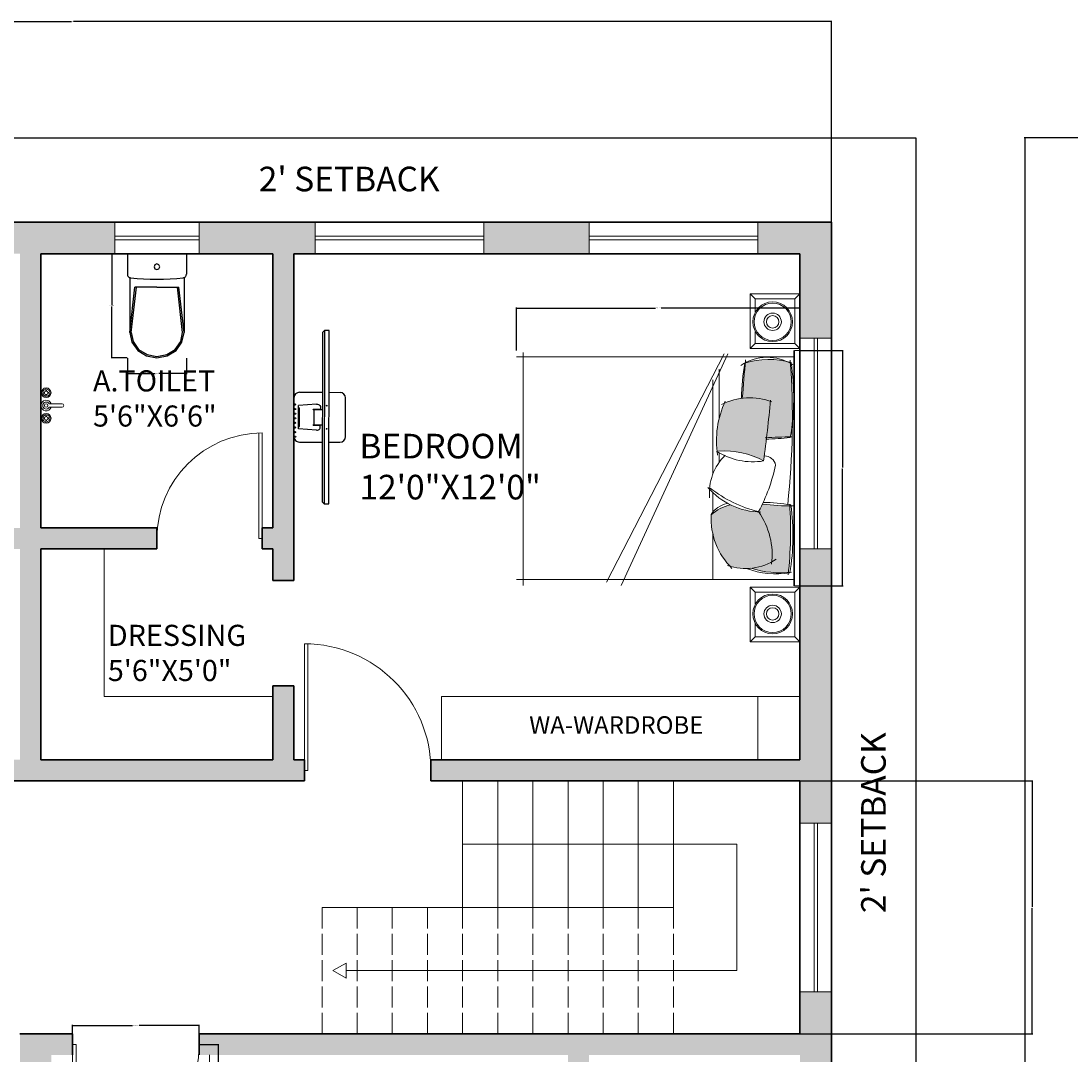
# Model space of a CAD drawing. Units: inches. Extents: x 3386 to 4477, y 1118 to 1824.
# Tile 5 of 7: x 3645 to 3944, y 1530 to 1824. Entities that reach past the tile are written whole.
import ezdxf

# ---------------------------------------------------------------- set-up
doc = ezdxf.new("R2010")
doc.units = ezdxf.units.IN
doc.linetypes.add('ACAD_ISO02W100', pattern=[15, 12, -3])
for name, color, linetype, lineweight in [('0.10', 252, 'Continuous', 9), ('0.15', 34, 'Continuous', 15), ('A-ANNO-DIMS', 2, 'Continuous', 18), ('A-ANNO-SYMB', 7, 'Continuous', 18), ('A-ANNO-TEXT', 7, 'Continuous', 18), ('A-AREA-IDEN', 7, 'Continuous', 18), ('A-DOOR', 4, 'Continuous', 18), ('A-EQPM', 9, 'Continuous', 18), ('A-FLOR-CASE', 7, 'Continuous', 18), ('A-FLOR-STRS', 7, 'Continuous', 18), ('A-FLOR-STRS-HIDN', 7, 'ACAD_ISO02W100', 13), ('A-FURN', 8, 'Continuous', 18), ('A-GLAZ', 4, 'Continuous', 18), ('A-WALL', 7, 'Continuous', 35), ('C-PROP', 7, 'Continuous', 25), ('Сантехника', 7, 'Continuous', 18)]:
    doc.layers.add(name, color=color, linetype=linetype, lineweight=lineweight)
doc.layers.add('A-FURN-PATT', color=116, linetype='Continuous', lineweight=13, true_color=0x136734)
doc.layers.add('A-WALL-PATT', color=18, linetype='Continuous', lineweight=13, true_color=0x000000)
doc.layers.add('SANTEH', color=7, linetype='Continuous')
doc.layers.add('window', color=130, linetype='Continuous')
doc.styles.get("Standard").update_dxf_attribs({"font": 'arial.ttf'})
doc.dimstyles.get("Standard").update_dxf_attribs({"dimtxt": 0.18, "dimasz": 0.18, "dimexe": 0.18, "dimexo": 0.0625, "dimgap": 0.09, "dimtad": 0, "dimtih": 1, "dimtoh": 1, "dimdec": 4, "dimzin": 0, "dimdsep": 46, "dimtxsty": 'Standard', "dimcen": 0.09, "dimadec": 0, "dimazin": 0, "dimtfac": 1, "dimtdec": 4, "dimtofl": 0, "dimtmove": 0, "dimatfit": 3, "dimfxl": 1, "dimtolj": 1, "dimtzin": 0, "dimarcsym": 0})

# ---------------------------------------------------------------- blocks, each defined once
blk = doc.blocks.new('D1')
for p, q in [((0, 36), (0, 0)), ((1, 36), (1, 0)), ((0, 0), (1, 0))]:
    blk.add_line(p, q)
blk.add_arc((0, 0), 36, 0, 90)
blk = doc.blocks.new('D2')
for p, q in [((0, 30), (0, 0)), ((1, 30), (1, 0)), ((0, 0), (1, 0))]:
    blk.add_line(p, q)
blk.add_arc((0, 0), 30, 0, 90)
blk = doc.blocks.new('WC 2 Symb_109')
at = {"layer": 'SANTEH'}
for p, q in [((0, 0), (0, 380)), ((0, 380), (132.4, 380)), ((153.6, 364.9), (506.8, 364.9)), ((506.3, 364.9), (215.7, 330.9)), ((506.3, 356), (215.7, 322)), ((215.7, 190), (215.7, 330.9)), ((215.7, 190), (215.7, 49.1)), ((153.8, 15.1), (506.8, 15.1)), ((506.3, 24), (215.7, 58)), ((506.3, 15.1), (215.7, 49.1)), ((0, 0), (132.4, 0))]:
    blk.add_line(p, q, dxfattribs=at)
for points in [[(154.6, 360.1), (153.9, 364.1), (152.3, 367.9), (150.2, 371.3), (147.4, 374.3), (144.1, 376.7), (140.5, 378.5), (136.5, 379.6), (132.4, 380)], [(154.6, 19.7), (158.6, 62.1), (161.4, 104.7), (163.1, 147.3), (163.7, 189.9), (163.1, 232.5), (161.4, 275.1), (158.6, 317.7), (154.6, 360.1)], [(506.3, 24), (565.5, 36.6), (615.7, 72.6), (649.2, 126.5), (661, 190), (649.2, 253.5), (615.7, 307.4), (565.5, 343.4), (506.3, 356)], [(506.8, 15.1), (569.2, 28.4), (622.2, 66.3), (657.6, 123.1), (670, 190), (657.6, 256.9), (622.2, 313.7), (569.2, 351.6), (506.8, 364.9)], [(132.4, 0), (136.5, 0.4), (140.4, 1.5), (144.1, 3.2), (147.3, 5.6), (150.1, 8.6), (152.3, 12), (153.8, 15.7), (154.6, 19.7)]]:
    blk.add_lwpolyline(points, dxfattribs=at)
blk.add_lwpolyline([(83.6, 208.5), (70.4, 203.1), (64.9, 190), (70.4, 176.9), (83.6, 171.5), (96.8, 176.9), (102.2, 190), (96.8, 203.1)], close=True, dxfattribs=at)
blk = doc.blocks.new('Faucet - Bathroom top')
for p, q in [((-4.107, 0.125), (-4.375, 0.125)), ((-3.75, 0.4788), (-3.75, 0.75)), ((-3.5, 0.482), (-3.5, 0.75)), ((-3.1461, 0.125), (-2.875, 0.125)), ((3.143, 0.125), (2.875, 0.125)), ((3.5, 0.4788), (3.5, 0.75)), ((3.75, 0.482), (3.75, 0.75)), ((4.1039, 0.125), (4.375, 0.125)), ((-4.1039, -0.125), (-4.375, -0.125)), ((-3.75, -0.4821), (-3.75, -0.75)), ((-3.5, -0.4789), (-3.5, -0.75)), ((-3.143, -0.125), (-2.875, -0.125)), ((-0.5, -0.8639), (-0.5, -4.5)), ((0.5, -4.5), (0.5, -0.8631)), ((3.1461, -0.125), (2.875, -0.125)), ((3.5, -0.4821), (3.5, -0.75)), ((3.75, -0.4789), (3.75, -0.75)), ((4.107, -0.125), (4.375, -0.125))]:
    blk.add_line(p, q)
for centre, radius in [((-3.625, 0), 1.375), ((-4.625, 0), 0.2795), ((-3.625, 0), 0.5), ((-3.625, 1), 0.2795), ((-2.625, 0), 0.2795), ((0, 0), 0.5), ((3.625, 0), 1.375), ((2.625, 0), 0.2795), ((3.625, 0), 0.5), ((3.625, 1), 0.2795), ((4.625, 0), 0.2795), ((-3.625, -1), 0.2795), ((3.625, -1), 0.2795)]:
    blk.add_circle(centre, radius)
for centre, radius, start, end in [((-3.625, 0), 1, 105.2407, 164.2093), ((-3.625, 0), 1, 16.44125, 74.07887), ((0, 0), 1.5, 289.6514, 250.3603), ((0, 0), 1, 300.3431, 239.7554), ((3.625, 0), 1, 106.12, 164.0884), ((3.625, 0), 1, 16.23422, 73.90469), ((-3.625, 0), 1, 196.2342, 253.9047), ((-3.625, 0), 1, 286.12, 344.0884), ((3.625, 0), 1, 196.4413, 254.0789), ((3.625, 0), 1, 285.2407, 344.2093), ((0, -4.5), 0.5, 180, 0)]:
    blk.add_arc(centre, radius, start, end)
blk = doc.blocks.new('TV')
at = {"color": 0}
for p, q in [((3967.27, 1784.85), (3967.05, 1784.65)), ((3967.76, 1763.68), (3967.54, 1763.86))]:
    blk.add_line(p, q, dxfattribs=at)
at = {"layer": 'window'}
for p, q in [((3967.54, 1763.86), (3967.05, 1784.65)), ((3964.41, 1777.23), (3967.22, 1777.3)), ((3968.01, 1777.32), (3969.36, 1777.35)), ((3966.53, 1775.82), (3964.33, 1775.61)), ((3964.34, 1775.34), (3964.45, 1775.34)), ((3964.34, 1775.31), (3964.43, 1775.32)), ((3966.14, 1775.2), (3967.01, 1775.22)), ((3966.14, 1775.18), (3967.27, 1775.2)), ((3966.14, 1775.18), (3966.14, 1775.2)), ((3966.3, 1773.29), (3966.26, 1775.18)), ((3964.39, 1773.06), (3964.48, 1773.06)), ((3966.19, 1773.28), (3967.31, 1773.31)), ((3966.19, 1773.26), (3967.05, 1773.28)), ((3966.19, 1773.26), (3966.19, 1773.28)), ((3964.39, 1773.04), (3964.5, 1773.04)), ((3966.61, 1772.66), (3964.4, 1772.77)), ((3964.55, 1771.15), (3967.36, 1771.22)), ((3968.15, 1771.24), (3969.5, 1771.27))]:
    blk.add_line(p, q, dxfattribs=at)
for points in [[(3968.33, 1763.69), (3967.83, 1784.86), (3967.27, 1784.85), (3967.76, 1763.68), (3968.33, 1763.69)], [(3963.86, 1771.81), (3963.75, 1776.54)], [(3970.16, 1771.96), (3970.05, 1776.69)], [(3964.4, 1772.77), (3964.33, 1775.61)], [(3964.48, 1773.06), (3964.43, 1775.32)], [(3964.5, 1773.04), (3964.45, 1775.34)]]:
    blk.add_lwpolyline(points, dxfattribs=at)
for points in [[(3966.53, 1775.82, -0.263666), (3966.93, 1775.69), (3967, 1775.57), (3967.01, 1775.22)], [(3966.61, 1772.66, 0.263666), (3967, 1772.81), (3967.06, 1772.93), (3967.05, 1773.28)]]:
    blk.add_lwpolyline(points, format="xyb", dxfattribs=at)
for centre, radius in [((3963.91, 1775.73), 0.0679), ((3967.77, 1775.68), 0.0451), ((3963.93, 1775.17), 0.0679), ((3963.94, 1774.6), 0.0679), ((3963.95, 1774.04), 0.0679), ((3963.97, 1773.48), 0.0679), ((3963.98, 1772.92), 0.0679), ((3963.99, 1772.35), 0.0679), ((3964.01, 1771.79), 0.0679), ((3967.83, 1772.86), 0.0451)]:
    blk.add_circle(centre, radius, dxfattribs=at)
for centre, start, end in [((3964.42, 1776.56), 91.3414, 181.3414), ((3969.38, 1776.67), 1.3414, 91.3414), ((3964.53, 1771.83), 181.3414, 271.3414), ((3969.49, 1771.94), 271.3414, 1.3414)]:
    blk.add_arc(centre, 0.676, start, end, dxfattribs=at)
blk = doc.blocks.new('camita')
at = {"layer": '0.10'}
for p, q in [((-0.85, -0.045), (0.85, -0.045)), ((-0.805, -0.045), (-0.805, -2.0485)), ((0.805, -0.045), (0.805, -2.0485)), ((-0.8271, -0.521), (0.8464, -1.2932)), ((-0.8271, -0.5476), (0.8236, -1.3992)), ((-0.7161, -0.585), (-0.3554, -0.585)), ((-0.1136, -0.585), (-0.0485, -0.585)), ((-0.638, -0.63), (0.0434, -0.63)), ((0.1749, -0.63), (0.3179, -0.63)), ((0.4739, -0.63), (0.805, -0.63)), ((-0.8354, -2), (0.8464, -2))]:
    blk.add_line(p, q, dxfattribs=at)
blk.add_lwpolyline([(-0.85, -0.0405), (0.85, -0.0405), (0.85, 0), (-0.85, 0)], close=True, dxfattribs=at)
for centre, radius, start, end in [((-0.4574, -0.2364), 0.3443, 147.50996, 213.83359), ((-0.1997, -0.2266), 0.5864, 163.92635, 197.14087), ((-0.3639, -5.8457), 5.7909, 83.80731, 94.12107), ((-0.5104, -1.7232), 1.6781, 80.12554, 98.66187), ((2.3534, -0.0532), 2.5803, 180.10628, 184.38541), ((-1.5443, -0.2452), 1.3333, 359.93941, 7.55329), ((1.5815, -0.2893), 1.3353, 170.38021, 178.99138), ((-1.4396, -0.0609), 1.7117, 352.92911, 0.39592), ((0.4524, -3.0675), 2.9996, 83.90257, 93.67595), ((0.4863, -1.6286), 1.5781, 80.16015, 98.05996), ((0.0294, -0.1377), 0.7262, 342.58415, 6.00484), ((0.1326, -0.1696), 0.6307, 339.92303, 8.74334), ((-0.0543, -0.3633), 0.4542, 159.30257, 206.50263), ((-1.3301, -9.6748), 9.4985, 82.27078, 84.93989), ((-0.007, -0.258), 0.0828, 100.01798, 179.73597), ((-0.2931, -1.4378), 1.2903, 61.97485, 77.84351), ((0.6265, -0.7518), 0.5508, 82.96906, 124.67388), ((0.3203, -0.3944), 0.4043, 341.45245, 33.45121), ((0.4585, -0.5454), 0.5842, 151.04555, 184.14969), ((-0.5341, -0.3393), 0.4875, 327.26442, 9.0473), ((-0.1986, -0.2742), 0.5159, 310.73945, 359.05759), ((-0.5673, -0.0868), 0.9057, 321.69527, 346.46261), ((-1.8672, -14.986), 14.6323, 84.65974, 85.75157), ((-0.4598, 1.4861), 1.9092, 260.95299, 268.65169), ((0.4384, -0.4834), 0.1898, 193.68485, 236.70352), ((0.5707, -0.4317), 0.3145, 192.93877, 221.96363), ((0.3612, -0.133), 0.5096, 267.25889, 315.29965), ((-0.2002, 0.064), 0.6673, 244.78094, 279.06058), ((0.179, -0.272), 0.3828, 224.52836, 275.22287)]:
    blk.add_arc(centre, radius, start, end, dxfattribs=at)
blk = doc.blocks.new('VELADOR')
at = {"layer": '0.15'}
for p, q in [((-0.2475, 0), (-0.2025, -0.045)), ((0.2475, 0), (0.2025, -0.045)), ((-0.2025, -0.405), (-0.2475, -0.45)), ((0.2475, -0.45), (0.2025, -0.405))]:
    blk.add_line(p, q, dxfattribs=at)
blk.add_lwpolyline([(-0.2475, 0), (-0.2475, -0.45), (0.2475, -0.45), (0.2475, 0)], close=True, dxfattribs=at)
blk.add_lwpolyline([(0.0921, -0.405), (0.2025, -0.405), (0.2025, -0.045), (-0.2025, -0.045), (-0.2025, -0.405), (-0.0818, -0.405)], dxfattribs=at)
for radius in [0.18, 0.1688, 0.0788, 0.0563]:
    blk.add_circle((0.0052, -0.2474), radius, dxfattribs=at)
blk = doc.blocks.new('WIN-24IN')
for p, q in [((0, 0), (0, 9)), ((24, 0), (24, 9)), ((0, 5), (24, 5)), ((0, 4), (24, 4))]:
    blk.add_line(p, q)
blk = doc.blocks.new('WIN-48IN')
for p, q in [((0, 48), (9, 48)), ((4, 0), (4, 48)), ((5, 0), (5, 48)), ((0, 0), (9, 0))]:
    blk.add_line(p, q)
blk = doc.blocks.new('WIN-60IN')
for p, q in [((0, 60), (9, 60)), ((4, 60), (4, 0)), ((5, 60), (5, 0)), ((0, 0), (9, 0))]:
    blk.add_line(p, q)
blk = doc.blocks.new('STAIR-DIRECTION')
blk.add_lwpolyline([(36.88, 38.16), (114.88, 38.16), (114.88, 2.16), (3.74, 2.16)])
blk.add_lwpolyline([(0, 2.16), (3.74, 0), (3.74, 4.32)], close=True)
blk = doc.blocks.new('WARDROBE-102IN')
for q in [(0, 18), (102, 0)]:
    blk.add_line((0, 0), q)
blk = doc.blocks.new('WARDROBE-102IN-DIVIDED')
for p, q in [((0, 18), (102, 18)), ((0, 0), (0, 18)), ((90, 18), (90, 0))]:
    blk.add_line(p, q)
blk = doc.blocks.new('DRESSING-UNIT-48X42')
for q in [(0, 42), (48, 0)]:
    blk.add_line((0, 0), q)
blk = doc.blocks.new('*D65')
at = {"layer": 'A-ANNO-DIMS', "color": 0, "lineweight": -2, "transparency": 16777216}
for p, q in [((3659.66, 1532.93), (3659.66, 1538.45)), ((3659.84, 1538.27), (3676.72, 1538.27)), ((3695.48, 1538.27), (3678.59, 1538.27)), ((3695.66, 1532.93), (3695.66, 1538.45))]:
    blk.add_line(p, q, dxfattribs=at)
at = {"layer": 'A-ANNO-DIMS', "color": 0, "transparency": 16777216}
for points in [[(3659.84, 1538.3), (3659.84, 1538.24), (3659.66, 1538.27)], [(3695.48, 1538.3), (3695.48, 1538.24), (3695.66, 1538.27)]]:
    blk.add_solid(points, dxfattribs=at)
at = {"layer": 'Defpoints', "color": 0, "transparency": 16777216}
for p in [(3695.66, 1538.27), (3659.66, 1532.87), (3695.66, 1532.87)]:
    blk.add_point(p, dxfattribs=at)
at = {"layer": 'A-ANNO-DIMS', "color": 0, "transparency": 16777216, "insert": (3677.66, 1538.27), "char_height": 0.18, "attachment_point": 5}
blk.add_mtext('\\A1;DOOR 36 TYP.', dxfattribs=at)
blk = doc.blocks.new('*D66')
at = {"layer": 'A-ANNO-DIMS', "color": 0, "lineweight": -2, "transparency": 16777216}
for p, q in [((3695.72, 1532.87), (3701.24, 1532.87)), ((3701.06, 1532.69), (3701.06, 1515.05)), ((3701.06, 1497.05), (3701.06, 1514.69)), ((3695.72, 1496.87), (3701.24, 1496.87))]:
    blk.add_line(p, q, dxfattribs=at)
at = {"layer": 'A-ANNO-DIMS', "color": 0, "transparency": 16777216}
for points in [[(3701.03, 1532.69), (3701.09, 1532.69), (3701.06, 1532.87)], [(3701.03, 1497.05), (3701.09, 1497.05), (3701.06, 1496.87)]]:
    blk.add_solid(points, dxfattribs=at)
at = {"layer": 'Defpoints', "color": 0, "transparency": 16777216}
for p in [(3695.66, 1532.87), (3695.66, 1496.87), (3701.06, 1496.87)]:
    blk.add_point(p, dxfattribs=at)
at = {"layer": 'A-ANNO-DIMS', "color": 0, "transparency": 16777216, "insert": (3701.06, 1514.87), "char_height": 0.18, "attachment_point": 5}
blk.add_mtext('\\A1;36 TYP.', dxfattribs=at)
blk = doc.blocks.new('*D77')
at = {"layer": 'A-ANNO-DIMS', "color": 0, "lineweight": -2, "transparency": 16777216}
for p, q in [((3675.2, 1757.87), (3670.64, 1757.87)), ((3670.82, 1757.69), (3670.82, 1743.25)), ((3670.82, 1728.44), (3670.82, 1742.88)), ((3675.2, 1728.26), (3670.64, 1728.26))]:
    blk.add_line(p, q, dxfattribs=at)
at = {"layer": 'A-ANNO-DIMS', "color": 0, "transparency": 16777216}
for points in [[(3670.79, 1757.69), (3670.85, 1757.69), (3670.82, 1757.87)], [(3670.79, 1728.44), (3670.85, 1728.44), (3670.82, 1728.26)]]:
    blk.add_solid(points, dxfattribs=at)
at = {"layer": 'Defpoints', "color": 0, "transparency": 16777216}
for p in [(3675.26, 1757.87), (3670.82, 1728.26), (3675.26, 1728.26)]:
    blk.add_point(p, dxfattribs=at)
at = {"layer": 'A-ANNO-DIMS', "color": 0, "transparency": 16777216, "insert": (3670.82, 1743.06), "char_height": 0.18, "attachment_point": 5}
blk.add_mtext('\\A1;WC 30 TYP.', dxfattribs=at)
blk = doc.blocks.new('*D78')
at = {"layer": 'A-ANNO-DIMS', "color": 0, "lineweight": -2, "transparency": 16777216}
for p, q in [((3675.26, 1728.2), (3675.26, 1723.64)), ((3692.05, 1728.2), (3692.05, 1723.64)), ((3675.44, 1723.82), (3683.14, 1723.82)), ((3691.87, 1723.82), (3684.17, 1723.82))]:
    blk.add_line(p, q, dxfattribs=at)
at = {"layer": 'A-ANNO-DIMS', "color": 0, "transparency": 16777216}
for points in [[(3675.44, 1723.85), (3675.44, 1723.79), (3675.26, 1723.82)], [(3691.87, 1723.85), (3691.87, 1723.79), (3692.05, 1723.82)]]:
    blk.add_solid(points, dxfattribs=at)
at = {"layer": 'Defpoints', "color": 0, "transparency": 16777216}
for p in [(3675.26, 1728.26), (3692.05, 1728.26), (3692.05, 1723.82)]:
    blk.add_point(p, dxfattribs=at)
at = {"layer": 'A-ANNO-DIMS', "color": 0, "transparency": 16777216, "insert": (3683.66, 1723.82), "char_height": 0.18, "attachment_point": 5}
blk.add_mtext('\\A1;17 TYP.', dxfattribs=at)
blk = doc.blocks.new('*D83')
at = {"layer": 'A-ANNO-DIMS', "color": 0, "lineweight": -2, "transparency": 16777216}
for p, q in [((3786, 1730.37), (3786, 1742.58)), ((3786.18, 1742.4), (3825.51, 1742.4)), ((3866.48, 1742.4), (3827.14, 1742.4)), ((3866.66, 1730.37), (3866.66, 1742.58))]:
    blk.add_line(p, q, dxfattribs=at)
at = {"layer": 'A-ANNO-DIMS', "color": 0, "transparency": 16777216}
for points in [[(3786.18, 1742.43), (3786.18, 1742.37), (3786, 1742.4)], [(3866.48, 1742.43), (3866.48, 1742.37), (3866.66, 1742.4)]]:
    blk.add_solid(points, dxfattribs=at)
at = {"layer": 'Defpoints', "color": 0, "transparency": 16777216}
for p in [(3866.66, 1742.4), (3786, 1730.3), (3866.66, 1730.3)]:
    blk.add_point(p, dxfattribs=at)
at = {"layer": 'A-ANNO-DIMS', "color": 0, "transparency": 16777216, "insert": (3826.33, 1742.4), "char_height": 0.18, "attachment_point": 5}
blk.add_mtext('\\A1;BED 81 TYP.', dxfattribs=at)
blk = doc.blocks.new('*D84')
at = {"layer": 'A-ANNO-DIMS', "color": 0, "lineweight": -2, "transparency": 16777216}
for p, q in [((3866.72, 1730.3), (3878.93, 1730.3)), ((3878.75, 1730.12), (3878.75, 1697.02)), ((3878.75, 1663.55), (3878.75, 1696.65)), ((3866.72, 1663.37), (3878.93, 1663.37))]:
    blk.add_line(p, q, dxfattribs=at)
at = {"layer": 'A-ANNO-DIMS', "color": 0, "transparency": 16777216}
for points in [[(3878.72, 1730.12), (3878.78, 1730.12), (3878.75, 1730.3)], [(3878.72, 1663.55), (3878.78, 1663.55), (3878.75, 1663.37)]]:
    blk.add_solid(points, dxfattribs=at)
at = {"layer": 'Defpoints', "color": 0, "transparency": 16777216}
for p in [(3866.66, 1730.3), (3866.66, 1663.37), (3878.75, 1663.37)]:
    blk.add_point(p, dxfattribs=at)
at = {"layer": 'A-ANNO-DIMS', "color": 0, "transparency": 16777216, "insert": (3878.75, 1696.83), "char_height": 0.18, "attachment_point": 5}
blk.add_mtext('\\A1;67 TYP.', dxfattribs=at)
blk = doc.blocks.new('*D103')
at = {"layer": 'A-ANNO-DIMS', "color": 0, "lineweight": -2, "transparency": 16777216}
for p, q in [((3443.66, 1745.93), (3443.66, 1824.1)), ((3443.84, 1823.92), (3659.36, 1823.92)), ((3875.48, 1823.92), (3659.95, 1823.92)), ((3875.66, 1766.93), (3875.66, 1824.1))]:
    blk.add_line(p, q, dxfattribs=at)
at = {"layer": 'A-ANNO-DIMS', "color": 0, "transparency": 16777216}
for points in [[(3443.84, 1823.95), (3443.84, 1823.89), (3443.66, 1823.92)], [(3875.48, 1823.95), (3875.48, 1823.89), (3875.66, 1823.92)]]:
    blk.add_solid(points, dxfattribs=at)
at = {"layer": 'Defpoints', "color": 0, "transparency": 16777216}
for p in [(3875.66, 1823.92), (3875.66, 1766.87), (3443.66, 1745.87)]:
    blk.add_point(p, dxfattribs=at)
at = {"layer": 'A-ANNO-DIMS', "color": 0, "transparency": 16777216, "insert": (3659.66, 1823.92), "char_height": 0.18, "attachment_point": 5}
blk.add_mtext('\\A1;432', dxfattribs=at)
blk = doc.blocks.new('*D104')
at = {"layer": 'A-ANNO-DIMS', "color": 0, "lineweight": -2, "transparency": 16777216}
for p, q in [((3866.72, 1607.87), (3932.89, 1607.87)), ((3932.71, 1607.69), (3932.71, 1572.05)), ((3932.71, 1536.05), (3932.71, 1571.69)), ((3866.72, 1535.87), (3932.89, 1535.87))]:
    blk.add_line(p, q, dxfattribs=at)
at = {"layer": 'A-ANNO-DIMS', "color": 0, "transparency": 16777216}
for points in [[(3932.68, 1607.69), (3932.74, 1607.69), (3932.71, 1607.87)], [(3932.68, 1536.05), (3932.74, 1536.05), (3932.71, 1535.87)]]:
    blk.add_solid(points, dxfattribs=at)
at = {"layer": 'Defpoints', "color": 0, "transparency": 16777216}
for p in [(3866.66, 1607.87), (3932.71, 1607.87), (3866.66, 1535.87)]:
    blk.add_point(p, dxfattribs=at)
at = {"layer": 'A-ANNO-DIMS', "color": 0, "transparency": 16777216, "insert": (3932.71, 1571.87), "char_height": 0.18, "attachment_point": 5}
blk.add_mtext('\\A1;72', dxfattribs=at)
blk = doc.blocks.new('*D106')
at = {"layer": 'A-ANNO-DIMS', "color": 0, "lineweight": -2, "transparency": 16777216}
for p, q in [((3963.65, 1790.87), (3930.48, 1790.87)), ((3930.66, 1790.69), (3930.66, 1491.05)), ((3930.66, 1191.05), (3930.66, 1490.69)), ((3963.65, 1190.87), (3930.48, 1190.87))]:
    blk.add_line(p, q, dxfattribs=at)
at = {"layer": 'A-ANNO-DIMS', "color": 0, "transparency": 16777216}
for points in [[(3930.63, 1790.69), (3930.69, 1790.69), (3930.66, 1790.87)], [(3930.63, 1191.05), (3930.69, 1191.05), (3930.66, 1190.87)]]:
    blk.add_solid(points, dxfattribs=at)
at = {"layer": 'Defpoints', "color": 0, "transparency": 16777216}
for p in [(3930.66, 1790.87), (3963.71, 1790.87), (3963.71, 1190.87)]:
    blk.add_point(p, dxfattribs=at)
at = {"layer": 'A-ANNO-DIMS', "color": 0, "transparency": 16777216, "insert": (3930.66, 1490.87), "char_height": 0.18, "attachment_point": 5}
blk.add_mtext('\\A1;600', dxfattribs=at)

msp = doc.modelspace()

# ---------------------------------------------------------------- hatches: boundary and pattern name
at = {"layer": 'A-FURN-PATT'}
h = msp.add_hatch(color=256, dxfattribs=at)
h.dxf.hatch_style = 1
h.paths.add_polyline_path([(3850.23, 1716.73, -0.113891), (3858.22, 1715.87, -0.006967), (3857.15, 1705.5, -0.016701), (3863.93, 1705.77, 0.015442), (3864.5, 1709.81, 0.01851), (3863.97, 1726.68, 0.020657), (3862.97, 1727.18, 0.131047), (3851.08, 1726.81, -0.004387)])
h.paths.add_polyline_path([(3855.96, 1686.63, -0.011742), (3854.89, 1684.5, -0.175864), (3858.65, 1670.19, -0.098488), (3852.71, 1668.38, 0.094792), (3863.39, 1667.16, 0.040212), (3863.77, 1686.12, -0.029051)])
h = msp.add_hatch(color=256, dxfattribs=at)
h.dxf.hatch_style = 1
h.paths.add_polyline_path([(3845.14, 1715.39, -0.189536), (3858.22, 1715.91, -0.011408), (3856.31, 1698.95, 0.150361), (3843.07, 1701.73, -0.133776)])
h.paths.add_polyline_path([(3858.64, 1670.24, -0.194952), (3846.75, 1668.96, -0.202559), (3841.37, 1683.62, -0.127326), (3846.88, 1686.48, 0.104045), (3854.98, 1684.41, -0.173835)])
at = {"layer": 'A-WALL-PATT'}
h = msp.add_hatch(color=256, dxfattribs=at)
h.dxf.hatch_style = 1
h.paths.add_polyline_path([(3443.66, 1221.87), (3452.66, 1221.87), (3452.66, 1301.87), (3458.66, 1301.87), (3458.66, 1310.87), (3452.66, 1310.87), (3452.66, 1328.87), (3443.66, 1328.87)])
h.paths.add_polyline_path([(3506.66, 1310.87), (3506.66, 1306.37), (3506.66, 1301.87), (3530.66, 1301.87), (3530.66, 1310.87)])
h.paths.add_polyline_path([(3653.66, 1301.87), (3653.66, 1382.87), (3662.66, 1382.87), (3662.66, 1391.87), (3653.66, 1391.87), (3653.66, 1529.87), (3659.66, 1529.87), (3659.66, 1535.87), (3644.66, 1535.87), (3644.66, 1310.87), (3602.66, 1310.87), (3602.66, 1301.87)])
h.paths.add_polyline_path([(3452.66, 1406.87), (3443.66, 1406.87), (3443.66, 1376.87), (3452.66, 1376.87), (3452.66, 1388.44)])
h.paths.add_polyline_path([(3452.66, 1478.87), (3452.66, 1502.87), (3478.74, 1502.87), (3482.66, 1502.87), (3482.66, 1504.87), (3482.66, 1517.87), (3473.66, 1517.87), (3473.66, 1511.87), (3443.66, 1511.87), (3443.66, 1478.87)])
h.paths.add_polyline_path([(3773.66, 1391.87), (3710.66, 1391.87), (3710.66, 1382.87), (3773.66, 1382.87)], flags=17)
h.paths.add_polyline_path([(3824.66, 1391.87), (3806.66, 1391.87), (3806.66, 1469.87), (3809.66, 1469.87), (3809.66, 1472.87), (3809.66, 1475.87), (3806.66, 1475.87), (3806.66, 1478.87), (3800.66, 1478.87), (3800.66, 1463.32), (3800.66, 1391.87), (3797.66, 1391.87), (3797.66, 1382.87), (3824.66, 1382.87)], flags=17)
h.paths.add_polyline_path([(3866.66, 1469.87), (3866.66, 1391.87), (3848.66, 1391.87), (3848.66, 1382.87), (3875.66, 1382.87), (3875.66, 1547.87), (3866.66, 1547.87), (3866.66, 1535.87), (3695.66, 1535.87), (3695.66, 1529.87), (3800.66, 1529.87), (3800.66, 1508.87), (3806.66, 1508.87), (3806.66, 1529.87), (3866.66, 1529.87), (3866.66, 1475.87), (3839.66, 1475.87), (3839.66, 1469.87)])
h.paths.add_polyline_path([(3875.66, 1673.87), (3866.66, 1673.87), (3866.66, 1663.37), (3866.66, 1647.44), (3866.66, 1613.87), (3761.66, 1613.87), (3761.66, 1607.87), (3866.66, 1607.87), (3866.66, 1595.87), (3875.66, 1595.87)])
h.paths.add_polyline_path([(3473.66, 1607.87), (3473.66, 1601.87), (3482.66, 1601.87), (3482.66, 1616.87), (3452.66, 1616.87), (3452.66, 1640.87), (3443.66, 1640.87), (3443.66, 1607.87)])
h.paths.add_polyline_path([(3491.66, 1736.87), (3491.66, 1745.87), (3478.95, 1745.87), (3443.66, 1745.87), (3443.66, 1688.87), (3452.66, 1688.87), (3452.66, 1736.87)])
h.paths.add_polyline_path([(3551.66, 1745.87), (3539.66, 1745.87), (3539.66, 1736.87), (3551.66, 1736.87)])
h.paths.add_polyline_path([(3587.66, 1745.87), (3581.66, 1745.87), (3581.66, 1741.37), (3581.66, 1736.87), (3587.66, 1736.87), (3587.66, 1712.87), (3596.66, 1712.87), (3596.66, 1757.87), (3644.66, 1757.87), (3644.66, 1679.87), (3596.66, 1679.87), (3596.66, 1682.87), (3592.16, 1682.87), (3587.66, 1682.87), (3587.66, 1607.87), (3602.66, 1607.87), (3602.66, 1613.87), (3596.66, 1613.87), (3596.66, 1673.87), (3644.66, 1673.87), (3644.66, 1613.87), (3638.66, 1613.87), (3638.66, 1610.87), (3638.66, 1607.87), (3725.66, 1607.87), (3725.66, 1613.87), (3722.66, 1613.87), (3722.66, 1634.87), (3716.66, 1634.87), (3716.66, 1613.87), (3650.66, 1613.87), (3650.66, 1673.87), (3683.66, 1673.87), (3683.66, 1679.87), (3650.66, 1679.87), (3650.66, 1757.87), (3671.66, 1757.87), (3671.66, 1766.87), (3587.66, 1766.87)])
h.paths.add_polyline_path([(3716.66, 1757.87), (3716.66, 1679.87), (3713.66, 1679.87), (3713.66, 1673.87), (3716.66, 1673.87), (3716.66, 1664.87), (3722.66, 1664.87), (3722.66, 1757.87), (3728.66, 1757.87), (3728.66, 1766.87), (3695.66, 1766.87), (3695.66, 1757.87)])
h.paths.add_polyline_path([(3806.66, 1757.87), (3806.66, 1766.87), (3776.66, 1766.87), (3776.66, 1757.87)])
h.paths.add_polyline_path([(3875.66, 1766.87), (3854.66, 1766.87), (3854.66, 1757.87), (3866.66, 1757.87), (3866.66, 1733.87), (3875.66, 1733.87)])

# ---------------------------------------------------------------- linework, layer by layer
at = {"layer": 'A-FLOR-STRS'}
for p, q in [((3770.66, 1607.87), (3770.66, 1571.87)), ((3780.66, 1607.87), (3780.66, 1571.87)), ((3790.66, 1607.87), (3790.66, 1571.87)), ((3800.66, 1607.87), (3800.66, 1571.87)), ((3810.66, 1607.87), (3810.66, 1571.87)), ((3820.66, 1607.87), (3820.66, 1571.87)), ((3830.66, 1607.87), (3830.66, 1571.87)), ((3730.66, 1571.87), (3830.66, 1571.87))]:
    msp.add_line(p, q, dxfattribs=at)
at = {"layer": 'A-FLOR-STRS-HIDN', "ltscale": 0.5}
for p, q in [((3730.66, 1571.87), (3730.66, 1535.87)), ((3740.66, 1571.87), (3740.66, 1535.87)), ((3750.66, 1571.87), (3750.66, 1535.87)), ((3760.66, 1571.87), (3760.66, 1535.87)), ((3770.66, 1571.87), (3770.66, 1535.87)), ((3780.66, 1571.87), (3780.66, 1535.87)), ((3790.66, 1571.87), (3790.66, 1535.87)), ((3800.66, 1571.87), (3800.66, 1535.87)), ((3810.66, 1571.87), (3810.66, 1535.87)), ((3820.66, 1571.87), (3820.66, 1535.87)), ((3830.66, 1571.87), (3830.66, 1535.87))]:
    msp.add_line(p, q, dxfattribs=at)
at = {"layer": 'A-WALL'}
for p, q in [((3587.66, 1766.87), (3875.66, 1766.87)), ((3875.66, 1766.87), (3875.66, 1382.87)), ((3650.66, 1679.87), (3650.66, 1757.87)), ((3650.66, 1757.87), (3716.66, 1757.87)), ((3716.66, 1757.87), (3716.66, 1679.87)), ((3722.66, 1757.87), (3722.66, 1664.87)), ((3722.66, 1757.87), (3866.66, 1757.87)), ((3866.66, 1757.87), (3866.66, 1613.87)), ((3650.66, 1679.87), (3683.66, 1679.87)), ((3683.66, 1679.87), (3683.66, 1673.87)), ((3713.66, 1679.87), (3713.66, 1673.87)), ((3713.66, 1679.87), (3716.66, 1679.87)), ((3650.66, 1613.87), (3650.66, 1673.87)), ((3650.66, 1673.87), (3683.66, 1673.87)), ((3713.66, 1673.87), (3716.66, 1673.87)), ((3716.66, 1673.87), (3716.66, 1664.87)), ((3716.66, 1664.87), (3722.66, 1664.87)), ((3716.66, 1634.87), (3722.66, 1634.87)), ((3716.66, 1634.87), (3716.66, 1613.87)), ((3722.66, 1634.87), (3722.66, 1613.87)), ((3650.66, 1613.87), (3716.66, 1613.87)), ((3722.66, 1613.87), (3725.66, 1613.87)), ((3725.66, 1613.87), (3725.66, 1607.87)), ((3761.66, 1613.87), (3761.66, 1607.87)), ((3761.66, 1613.87), (3866.66, 1613.87)), ((3638.66, 1607.87), (3725.66, 1607.87)), ((3761.66, 1607.87), (3866.66, 1607.87)), ((3866.66, 1607.87), (3866.66, 1535.87)), ((3644.66, 1535.87), (3659.66, 1535.87)), ((3659.66, 1529.87), (3659.66, 1535.87)), ((3695.66, 1529.87), (3695.66, 1535.87)), ((3695.66, 1535.87), (3866.66, 1535.87))]:
    msp.add_line(p, q, dxfattribs=at)
at = {"layer": 'C-PROP'}
msp.add_lwpolyline([(3419.66, 1790.87), (3899.66, 1790.87), (3899.66, 1190.87), (3419.66, 1190.87)], close=True, dxfattribs=at)

# ---------------------------------------------------------------- block references
at = {"layer": 'A-ANNO-SYMB'}
msp.add_blockref('STAIR-DIRECTION', (3733.77, 1551.71), dxfattribs=at)
at = {"layer": 'A-DOOR', "xscale": -1}
msp.add_blockref('D2', (3713.66, 1676.87), dxfattribs=at)
at = {"layer": 'A-DOOR'}
msp.add_blockref('D1', (3725.66, 1610.87), dxfattribs=at)
at = {"layer": 'A-DOOR', "xscale": -1, "rotation": 180}
msp.add_blockref('D1', (3659.66, 1532.87), dxfattribs=at)
at = {"layer": 'A-EQPM', "xscale": 2.327319231123021, "yscale": 2.327319231123021, "zscale": 2.327319231123021, "rotation": 358.5430845181613}
msp.add_blockref('TV', (-5604.37, -2181.82), dxfattribs=at)
at = {"layer": 'A-FLOR-CASE'}
for name, p in [('DRESSING-UNIT-48X42', (3668.66, 1631.87)), ('WARDROBE-102IN-DIVIDED', (3764.66, 1613.87)), ('WARDROBE-102IN', (3698.66, 1511.87))]:
    msp.add_blockref(name, p, dxfattribs=at)
at = {"layer": 'A-FURN'}
for name, p, xscale, yscale, zscale, rotation in [('VELADOR', (3866.66, 1738.67), 31.41542173157097, 31.41542173157097, 31.41542173157097, 270), ('camita', (3866.66, 1696.83), 39.375, 39.375, 39.375, 270), ('VELADOR', (3866.66, 1655.22), -31.41542173157097, 31.41542173157097, 31.41542173157097, 269.9999999999999)]:
    msp.add_blockref(name, p, dxfattribs=dict(at, xscale=xscale, yscale=yscale, zscale=zscale, rotation=rotation))
at = {"layer": 'A-GLAZ'}
for name, p in [('WIN-24IN', (3671.66, 1757.87)), ('WIN-60IN', (3866.66, 1673.87)), ('WIN-48IN', (3866.66, 1547.87))]:
    msp.add_blockref(name, p, dxfattribs=at)
for p, rotation in [((3776.66, 1757.87), 89.99999999999818), ((3806.66, 1766.87), 269.9999999999999)]:
    msp.add_blockref('WIN-48IN', p, dxfattribs=dict(at, rotation=rotation))
at = {"layer": 'Сантехника', "xscale": 0.0441898926459964, "yscale": 0.0441898926459964, "zscale": 0.0441898926459964, "rotation": 269.9999999999999}
msp.add_blockref('WC 2 Symb_109', (3675.26, 1757.87), dxfattribs=at)
at = {"layer": 'Сантехника', "rotation": 90}
msp.add_blockref('Faucet - Bathroom top', (3652.16, 1714.68), dxfattribs=at)

# ---------------------------------------------------------------- texts
at = {"layer": 'A-ANNO-TEXT', "attachment_point": 1}
for s, insert, char_height in [("{\\fTimes New Roman|b0|i0|c0|p18;2' SETBACK}", (3712.65, 1782.64), 7), ('{\\fTimes New Roman|b0|i0|c0|p18;WA-WARDROBE}', (3789.61, 1626.26), 5)]:
    msp.add_mtext_dynamic_manual_height_columns(s, width=79.5604, gutter_width=12.5, heights=[0], dxfattribs=dict(at, insert=insert, char_height=char_height))
at = {"layer": 'A-ANNO-TEXT', "insert": (3884.07, 1570.24), "char_height": 7, "attachment_point": 1, "rotation": 90}
msp.add_mtext_dynamic_manual_height_columns("{\\fTimes New Roman|b0|i0|c0|p18;2' SETBACK}", width=79.5604, gutter_width=12.5, heights=[0], dxfattribs=at)
at = {"layer": 'A-AREA-IDEN', "attachment_point": 1}
for s, width, insert, char_height in [('{\\fTimes New Roman|b0|i0|c0|p18;A.TOILET\\P5\'6"X6\'6"}', 79.5604, (3665.48, 1724.69), 6), ('{\\fTimes New Roman|b0|i0|c0|p18;BEDROOM\\P12\'0"X12\'0"}', 79.5604, (3741.3, 1706.63), 7), ('{\\fTimes New Roman|b0|i0|c0|p18;DRESSING\\P5\'6"X5\'0"}', 52.5784, (3669.71, 1652.28), 6)]:
    msp.add_mtext_dynamic_manual_height_columns(s, width=width, gutter_width=12.5, heights=[0], dxfattribs=dict(at, insert=insert, char_height=char_height))

# ---------------------------------------------------------------- dimensions: what is measured, and where the dimension line sits
at = {"layer": 'A-ANNO-DIMS'}
dim = msp.add_linear_dim(base=(3875.66, 1823.92), p1=(3443.66, 1745.87), p2=(3875.66, 1766.87), dimstyle='Standard', override={"dimdec": 0, "dimlfac": 1, "dimrnd": 0, "dimzin": 0, "dimdsep": 46, "dimlunit": 2}, dxfattribs=at)
dim.commit()
dim.dimension.update_dxf_attribs({"geometry": '*D103', "text_midpoint": (3659.66, 1823.92)})
for base, p1, p2, picture, middle in [((3930.66, 1790.87), (3963.71, 1190.87), (3963.71, 1790.87), '*D106', (3930.66, 1490.87)), ((3932.71, 1607.87), (3866.66, 1535.87), (3866.66, 1607.87), '*D104', (3932.71, 1571.87))]:
    dim = msp.add_linear_dim(base=base, p1=p1, p2=p2, angle=90, dimstyle='Standard', override={"dimdec": 0, "dimlfac": 1, "dimrnd": 0, "dimzin": 0, "dimdsep": 46, "dimlunit": 2}, dxfattribs=at)
    dim.commit()
    dim.dimension.update_dxf_attribs({"geometry": picture, "text_midpoint": middle})
for base, p1, p2, text, picture, middle in [((3670.82, 1728.26), (3675.26, 1757.87), (3675.26, 1728.26), 'WC <> TYP.', '*D77', (3670.82, 1743.06)), ((3878.75, 1663.37), (3866.66, 1730.3), (3866.66, 1663.37), '<> TYP.', '*D84', (3878.75, 1696.83)), ((3701.06, 1496.87), (3695.66, 1532.87), (3695.66, 1496.87), '<> TYP.', '*D66', (3701.06, 1514.87))]:
    dim = msp.add_linear_dim(base=base, p1=p1, p2=p2, angle=270, text=text, dimstyle='Standard', override={"dimdec": 0, "dimlfac": 1, "dimrnd": 0, "dimzin": 0, "dimdsep": 46, "dimlunit": 2}, dxfattribs=at)
    dim.commit()
    dim.dimension.update_dxf_attribs({"geometry": picture, "text_midpoint": middle})
for base, p1, p2, text, picture, middle in [((3866.66, 1742.4), (3786, 1730.3), (3866.66, 1730.3), 'BED <> TYP.', '*D83', (3826.33, 1742.4)), ((3692.05, 1723.82), (3675.26, 1728.26), (3692.05, 1728.26), '<> TYP.', '*D78', (3683.66, 1723.82)), ((3695.66, 1538.27), (3659.66, 1532.87), (3695.66, 1532.87), 'DOOR <> TYP.', '*D65', (3677.66, 1538.27))]:
    dim = msp.add_linear_dim(base=base, p1=p1, p2=p2, text=text, dimstyle='Standard', override={"dimdec": 0, "dimlfac": 1, "dimrnd": 0, "dimzin": 0, "dimdsep": 46, "dimlunit": 2}, dxfattribs=at)
    dim.commit()
    dim.dimension.update_dxf_attribs({"geometry": picture, "text_midpoint": middle})

doc.saveas('drawing.dxf')
